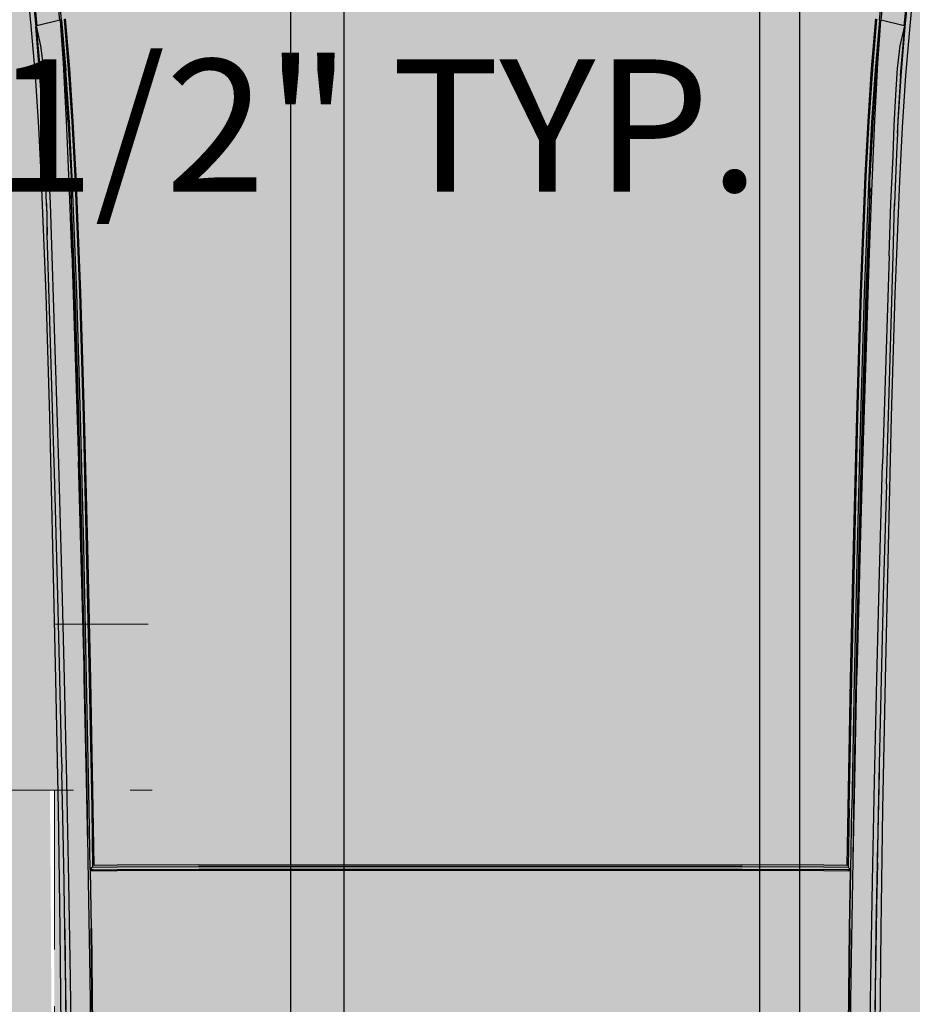
# Model space of a CAD drawing. Units: inches. Extents: x 1884 to 2398, y 474 to 1488.
# Tile 24 of 39: x 2301 to 2348, y 620 to 672. Entities that reach past the tile are written whole.
import ezdxf

# ---------------------------------------------------------------- set-up
doc = ezdxf.new("R2010")
doc.units = ezdxf.units.IN
doc.header["$MEASUREMENT"] = 0
doc.linetypes.add('ACAD_ISO02W100', pattern=[15, 12, -3])
doc.layers.get('0').update_dxf_attribs({"color": 250})
for name, color, linetype, lineweight in [('A-ANNO-DIMS', 2, 'Continuous', 18), ('A-FLOR-OVHD', 8, 'ACAD_ISO02W100', 18), ('C-VEHI', 8, 'Continuous', 18)]:
    doc.layers.add(name, color=color, linetype=linetype, lineweight=lineweight)
doc.layers.add('Edges', color=250, linetype='Continuous')
doc.layers.add('L-PVMT-PATT', color=9, linetype='Continuous', lineweight=13, true_color=0xc7c8ca)
doc.styles.get("Standard").update_dxf_attribs({"font": 'arial.ttf'})
doc.dimstyles.get("Standard").update_dxf_attribs({"dimtxt": 7, "dimasz": 0.18, "dimexe": 0.18, "dimexo": 0.0625, "dimgap": 0.09, "dimtad": 0, "dimtih": 1, "dimtoh": 1, "dimzin": 0, "dimdsep": 46, "dimlunit": 3, "dimtxsty": 'Standard', "dimcen": 0.09, "dimadec": 0, "dimazin": 0, "dimtfac": 1, "dimtofl": 0, "dimtmove": 0, "dimatfit": 3, "dimfxl": 1, "dimtolj": 1, "dimtzin": 0, "dimarcsym": 0})

# ---------------------------------------------------------------- blocks, each defined once
blk = doc.blocks.new('Nissan Qashqai pl')
at = {"layer": 'Edges'}
for p, q in [((9.2783, 12.5191), (9.3422, 12.5126)), ((9.3427, 12.5066), (9.2789, 12.5131)), ((9.3418, 12.5051), (9.2819, 12.5112)), ((9.3418, 12.5051), (9.3346, 12.4741)), ((9.342, 12.5059), (9.3418, 12.5051)), ((9.3687, 12.5), (9.342, 12.5059)), ((9.4087, 12.5003), (9.342, 12.5059)), ((9.3422, 12.5126), (9.4088, 12.507)), ((9.4093, 12.5011), (9.3427, 12.5066)), ((9.4088, 12.507), (9.4782, 12.5024)), ((9.4782, 12.5024), (9.5503, 12.4987)), ((9.3992, 12.496), (9.3687, 12.5)), ((9.4347, 12.494), (9.3992, 12.496)), ((9.4087, 12.5003), (9.4688, 12.4968)), ((9.4785, 12.4965), (9.4093, 12.5011)), ((9.4761, 12.4919), (9.4347, 12.494)), ((9.4688, 12.4968), (9.4789, 12.4964)), ((9.5168, 12.4903), (9.4761, 12.4919)), ((9.4789, 12.4964), (9.4785, 12.4965)), ((9.4862, 12.4961), (9.4785, 12.4965)), ((9.4789, 12.4964), (9.4862, 12.4961)), ((9.4862, 12.4961), (9.514, 12.4949)), ((9.514, 12.4949), (9.5811, 12.492)), ((9.5812, 12.4874), (9.5168, 12.4903)), ((9.5503, 12.4987), (9.7029, 12.4926)), ((9.651, 12.4906), (9.5811, 12.492)), ((9.5811, 12.492), (9.594, 12.4914)), ((9.9583, 12.4812), (9.651, 12.4906)), ((9.7029, 12.4926), (9.8673, 12.4878)), ((9.3346, 12.4718), (9.2704, 12.4783)), ((9.3346, 12.4741), (9.2724, 12.4804)), ((9.6514, 12.4849), (9.5812, 12.4874)), ((9.6514, 12.4849), (9.9312, 12.4761)), ((9.8673, 12.4878), (10.0423, 12.4835)), ((10.0776, 12.4719), (9.9312, 12.4761)), ((9.9583, 12.4812), (10.091, 12.4775)), ((10.0423, 12.4835), (10.2211, 12.4795)), ((10.091, 12.4775), (10.2202, 12.4743)), ((10.2211, 12.4795), (10.3955, 12.4762)), ((10.3955, 12.4762), (10.5572, 12.4737)), ((9.3326, 12.4666), (9.4, 12.4609)), ((9.4004, 12.4629), (9.333, 12.4685)), ((9.3346, 12.4741), (9.3344, 12.4733)), ((9.3344, 12.4733), (9.4017, 12.4677)), ((9.3344, 12.4733), (9.3611, 12.4715)), ((9.3346, 12.4718), (9.4018, 12.4661)), ((9.3611, 12.4715), (9.3918, 12.4695)), ((9.3918, 12.4695), (9.4276, 12.4674)), ((9.4709, 12.4581), (9.4004, 12.4629)), ((9.4017, 12.4677), (9.472, 12.463)), ((9.4018, 12.4661), (9.472, 12.4614)), ((9.4276, 12.4674), (9.4694, 12.4654)), ((9.4694, 12.4654), (9.5105, 12.4637)), ((9.472, 12.463), (9.5454, 12.4591)), ((9.5105, 12.4637), (9.5755, 12.4608)), ((10.2201, 12.4683), (10.0776, 12.4719)), ((10.3586, 12.4651), (10.2201, 12.4683)), ((10.2202, 12.4743), (10.2203, 12.4743)), ((10.2203, 12.4743), (10.3353, 12.4717)), ((10.3353, 12.4717), (10.4477, 12.4694)), ((10.3353, 12.4717), (10.346, 12.4714)), ((10.346, 12.4714), (10.4477, 12.4694)), ((10.4931, 12.4624), (10.3586, 12.4651)), ((10.4477, 12.4694), (10.4538, 12.4693)), ((10.4538, 12.4693), (10.4681, 12.469)), ((10.4676, 12.4691), (10.4538, 12.4693)), ((10.5566, 12.4677), (10.4676, 12.4691)), ((10.4676, 12.4691), (10.546, 12.4677)), ((10.4681, 12.469), (10.5866, 12.467)), ((10.6237, 12.4603), (10.4931, 12.4624)), ((10.546, 12.4677), (10.546, 12.4678)), ((10.546, 12.4677), (10.5576, 12.4675)), ((10.7, 12.4662), (10.5566, 12.4677)), ((10.5572, 12.4737), (10.7004, 12.4722)), ((10.5576, 12.4675), (10.6649, 12.4659)), ((10.5866, 12.467), (10.6649, 12.4659)), ((9.4, 12.4609), (9.4706, 12.4561)), ((9.4706, 12.4561), (9.5443, 12.4522)), ((9.5446, 12.4542), (9.4709, 12.4581)), ((9.472, 12.4614), (9.5454, 12.4576)), ((9.5443, 12.4522), (9.701, 12.4459)), ((9.7011, 12.4478), (9.5446, 12.4542)), ((9.5454, 12.4591), (9.5454, 12.4593)), ((9.5695, 12.4589), (9.5454, 12.4591)), ((9.5454, 12.4576), (9.7014, 12.4513)), ((9.5609, 12.4593), (9.5695, 12.4589)), ((9.5786, 12.4588), (9.5695, 12.4589)), ((9.5695, 12.4589), (9.7014, 12.4536)), ((9.5755, 12.4608), (9.6472, 12.4581)), ((9.6206, 12.4581), (9.5786, 12.4588)), ((9.6714, 12.4567), (9.6206, 12.4581)), ((9.6414, 12.458), (9.6407, 12.458)), ((9.6472, 12.4581), (9.9278, 12.4492)), ((9.6549, 12.4576), (9.6558, 12.4574)), ((9.6825, 12.4564), (9.6714, 12.4567)), ((9.6825, 12.4564), (9.6829, 12.4563)), ((9.6943, 12.456), (9.6825, 12.4564)), ((9.6943, 12.4558), (9.6943, 12.456)), ((9.6951, 12.456), (9.6943, 12.456)), ((9.6951, 12.4558), (9.6951, 12.456)), ((9.8565, 12.451), (9.6951, 12.456)), ((9.7014, 12.4536), (9.8673, 12.4488)), ((9.7014, 12.4513), (9.8673, 12.4464)), ((9.9794, 12.4475), (9.8565, 12.451)), ((9.8673, 12.4488), (10.0429, 12.4444)), ((9.9278, 12.4492), (10.0747, 12.445)), ((10.7502, 12.4586), (10.6237, 12.4603)), ((9.701, 12.4459), (9.8673, 12.441)), ((9.8673, 12.443), (9.7011, 12.4478)), ((9.8673, 12.4464), (10.0429, 12.4421)), ((10.043, 12.4387), (9.8673, 12.443)), ((9.8673, 12.441), (10.0431, 12.4367)), ((10.0998, 12.4443), (9.9794, 12.4475)), ((10.0429, 12.4444), (10.2216, 12.4404)), ((10.0429, 12.4421), (10.2215, 12.4381)), ((10.2218, 12.4347), (10.043, 12.4387)), ((10.0431, 12.4367), (10.2218, 12.4327)), ((10.0747, 12.445), (10.078, 12.4449)), ((10.078, 12.4449), (10.2146, 12.4414)), ((10.2146, 12.4414), (10.0998, 12.4443)), ((10.2146, 12.4414), (10.2175, 12.4413)), ((10.2175, 12.4413), (10.3564, 12.4382)), ((10.2215, 12.4381), (10.3945, 12.4348)), ((10.2216, 12.4404), (10.3947, 12.4371)), ((10.3564, 12.4382), (10.4638, 12.436)), ((10.3947, 12.4371), (10.4638, 12.436)), ((10.4638, 12.436), (10.4914, 12.4355)), ((10.4914, 12.4355), (10.6223, 12.4333)), ((10.3947, 12.4314), (10.2218, 12.4347)), ((10.2218, 12.4327), (10.3947, 12.4294)), ((10.4773, 12.4335), (10.3945, 12.4348)), ((10.3947, 12.4314), (10.4735, 12.4301)), ((10.3947, 12.4294), (10.4715, 12.4282)), ((10.4715, 12.4282), (10.4711, 12.3973)), ((10.4731, 12.3973), (10.4735, 12.4301)), ((10.4735, 12.4301), (10.4773, 12.4335)), ((10.4773, 12.4296), (10.4769, 12.3968)), ((10.4773, 12.4335), (10.4773, 12.4296)), ((10.4785, 12.433), (10.4773, 12.4335)), ((10.5561, 12.4323), (10.4773, 12.4335)), ((10.4781, 12.3972), (10.4785, 12.433)), ((10.5563, 12.4318), (10.4785, 12.433)), ((10.5561, 12.4323), (10.6996, 12.4308)), ((10.6999, 12.4304), (10.5563, 12.4318)), ((10.6223, 12.4333), (10.7493, 12.4316)), ((10.4711, 12.3973), (10.4706, 12.2875)), ((10.4726, 12.2875), (10.4731, 12.3973)), ((10.4764, 12.2872), (10.4769, 12.3968)), ((10.4776, 12.2874), (10.4781, 12.3972)), ((10.4706, 11.5566), (10.4706, 12.2875)), ((10.4726, 11.5567), (10.4726, 12.2875)), ((10.4764, 11.5569), (10.4764, 12.2872)), ((10.4776, 11.5567), (10.4776, 12.2874)), ((10.4706, 11.5566), (10.4711, 11.4469)), ((10.4731, 11.4469), (10.4726, 11.5567)), ((10.4769, 11.4474), (10.4764, 11.5569)), ((10.4781, 11.4469), (10.4776, 11.5567)), ((10.4711, 11.4469), (10.4715, 11.416)), ((10.4735, 11.414), (10.4731, 11.4469)), ((10.4773, 11.4146), (10.4769, 11.4474)), ((10.4785, 11.4111), (10.4781, 11.4469)), ((10.4715, 11.416), (10.3947, 11.4148)), ((9.8673, 11.4031), (9.701, 11.3983)), ((10.0431, 11.4075), (9.8673, 11.4031)), ((9.8673, 11.4012), (10.043, 11.4055)), ((10.2215, 11.406), (10.0429, 11.4021)), ((10.2216, 11.4037), (10.0429, 11.3998)), ((10.043, 11.4055), (10.2218, 11.4094)), ((10.2218, 11.4114), (10.0431, 11.4075)), ((10.2043, 11.4025), (10.0747, 11.3991)), ((10.0998, 11.3999), (10.2043, 11.4025)), ((10.2175, 11.4028), (10.2043, 11.4025)), ((10.3564, 11.406), (10.2175, 11.4028)), ((10.3945, 11.4094), (10.2215, 11.406)), ((10.3947, 11.4071), (10.2216, 11.4037)), ((10.3947, 11.4148), (10.2218, 11.4114)), ((10.2218, 11.4094), (10.3947, 11.4128)), ((10.4416, 11.4077), (10.3564, 11.406)), ((10.4773, 11.4107), (10.3945, 11.4094)), ((10.3947, 11.4128), (10.4735, 11.414)), ((10.4416, 11.4078), (10.3947, 11.4071)), ((10.4519, 11.4079), (10.4416, 11.4077)), ((10.4519, 11.4079), (10.4416, 11.4078)), ((10.4416, 11.4077), (10.4416, 11.4078)), ((10.4524, 11.408), (10.4519, 11.4079)), ((10.4519, 11.4079), (10.4519, 11.4079)), ((10.4524, 11.4079), (10.4519, 11.4079)), ((10.4524, 11.4079), (10.4524, 11.408)), ((10.4533, 11.408), (10.4524, 11.408)), ((10.4533, 11.4079), (10.4524, 11.4079)), ((10.4638, 11.4081), (10.4533, 11.4079)), ((10.4638, 11.4081), (10.4533, 11.408)), ((10.4533, 11.4079), (10.4533, 11.408)), ((10.4914, 11.4087), (10.4638, 11.4081)), ((10.4773, 11.4107), (10.4735, 11.414)), ((10.4773, 11.4146), (10.4773, 11.4107)), ((10.4773, 11.4107), (10.5561, 11.4119)), ((10.4773, 11.4107), (10.4785, 11.4111)), ((10.5563, 11.4123), (10.4785, 11.4111)), ((10.6223, 11.4109), (10.4914, 11.4087)), ((10.6996, 11.4134), (10.5561, 11.4119)), ((10.5563, 11.4123), (10.6999, 11.4138)), ((10.7493, 11.4125), (10.6223, 11.4109)), ((9.5443, 11.3919), (9.4706, 11.388)), ((9.4709, 11.3861), (9.5446, 11.39)), ((9.701, 11.3983), (9.5443, 11.3919)), ((9.5446, 11.39), (9.7011, 11.3963)), ((9.7014, 11.3929), (9.5454, 11.3866)), ((9.7014, 11.3906), (9.5695, 11.3853)), ((9.6472, 11.3861), (9.9278, 11.3949)), ((9.6714, 11.3874), (9.8565, 11.3931)), ((9.7011, 11.3963), (9.8673, 11.4012)), ((9.8673, 11.3977), (9.7014, 11.3929)), ((9.8673, 11.3954), (9.7014, 11.3906)), ((9.8565, 11.3931), (9.9794, 11.3967)), ((10.0429, 11.4021), (9.8673, 11.3977)), ((10.0429, 11.3998), (9.8673, 11.3954)), ((10.0747, 11.3991), (9.9278, 11.3949)), ((9.9794, 11.3967), (10.0965, 11.3998)), ((10.0965, 11.3998), (10.0998, 11.3999)), ((9.4, 11.3832), (9.3326, 11.3776)), ((9.333, 11.3757), (9.4004, 11.3813)), ((9.4017, 11.3765), (9.3344, 11.3708)), ((9.3346, 11.3724), (9.4018, 11.378)), ((9.4276, 11.3767), (9.3918, 11.3747)), ((9.4706, 11.388), (9.4, 11.3832)), ((9.4004, 11.3813), (9.4709, 11.3861)), ((9.472, 11.3812), (9.4017, 11.3765)), ((9.472, 11.3828), (9.4018, 11.378)), ((9.4694, 11.3788), (9.4276, 11.3767)), ((9.5105, 11.3805), (9.4694, 11.3788)), ((9.5454, 11.3866), (9.472, 11.3828)), ((9.472, 11.3812), (9.5454, 11.3851)), ((9.5755, 11.3834), (9.5105, 11.3805)), ((9.5454, 11.3851), (9.5695, 11.3853)), ((9.5454, 11.3848), (9.5454, 11.3851)), ((9.5695, 11.3853), (9.5609, 11.3849)), ((9.5695, 11.3853), (9.5786, 11.3853)), ((9.6472, 11.3861), (9.5755, 11.3834)), ((9.5786, 11.3853), (9.6206, 11.3861)), ((9.6206, 11.3861), (9.6714, 11.3874)), ((10.0776, 11.3722), (10.2201, 11.3759)), ((10.2201, 11.3759), (10.3586, 11.3791)), ((10.3586, 11.3791), (10.4931, 11.3817)), ((10.5576, 11.3766), (10.4676, 11.3751)), ((10.5566, 11.3765), (10.4676, 11.3751)), ((10.5866, 11.3772), (10.4681, 11.3752)), ((10.4931, 11.3817), (10.6237, 11.3839)), ((10.5566, 11.3765), (10.7, 11.378)), ((10.6649, 11.3783), (10.5576, 11.3766)), ((10.6649, 11.3783), (10.5866, 11.3772)), ((10.6237, 11.3839), (10.7502, 11.3855)), ((9.3346, 11.3724), (9.2704, 11.3659)), ((9.3346, 11.37), (9.2724, 11.3637)), ((9.3611, 11.3727), (9.3344, 11.3708)), ((9.3344, 11.3708), (9.3346, 11.37)), ((9.3346, 11.37), (9.3418, 11.3391)), ((9.3918, 11.3747), (9.3611, 11.3727)), ((9.9583, 11.363), (9.651, 11.3536)), ((9.6514, 11.3592), (9.9312, 11.3681)), ((9.9312, 11.3681), (10.0776, 11.3722)), ((10.091, 11.3666), (9.9583, 11.363)), ((10.2211, 11.3646), (10.0423, 11.3607)), ((10.2191, 11.3699), (10.091, 11.3666)), ((10.2202, 11.3699), (10.2191, 11.3699)), ((10.2202, 11.3699), (10.2203, 11.3699)), ((10.3353, 11.3725), (10.2203, 11.3699)), ((10.3955, 11.368), (10.2211, 11.3646)), ((10.3353, 11.3725), (10.346, 11.3727)), ((10.4477, 11.3747), (10.346, 11.3727)), ((10.5572, 11.3704), (10.3955, 11.368)), ((10.4537, 11.3749), (10.4477, 11.3747)), ((10.4537, 11.3749), (10.4538, 11.3749)), ((10.4681, 11.3752), (10.4538, 11.3749)), ((10.4676, 11.3751), (10.4538, 11.3749)), ((10.4676, 11.3751), (10.4676, 11.3751)), ((10.7004, 11.372), (10.5572, 11.3704)), ((9.3992, 11.3482), (9.4347, 11.3502)), ((9.4347, 11.3502), (9.4761, 11.3522)), ((9.4761, 11.3522), (9.5168, 11.3539)), ((9.5811, 11.3522), (9.514, 11.3492)), ((9.5168, 11.3539), (9.5812, 11.3568)), ((9.7029, 11.3516), (9.5503, 11.3455)), ((9.5811, 11.3522), (9.6231, 11.3531)), ((9.594, 11.3527), (9.5811, 11.3522)), ((9.5812, 11.3568), (9.6514, 11.3592)), ((9.6231, 11.3531), (9.594, 11.3527)), ((9.651, 11.3536), (9.6231, 11.3531)), ((9.8673, 11.3563), (9.7029, 11.3516)), ((10.0423, 11.3607), (9.8673, 11.3563)), ((9.2789, 11.331), (9.3427, 11.3375)), ((9.2819, 11.333), (9.3418, 11.3391)), ((9.3418, 11.3391), (9.342, 11.3383)), ((9.342, 11.3383), (9.3687, 11.3441)), ((9.342, 11.3383), (9.4087, 11.3438)), ((9.4088, 11.3371), (9.3422, 11.3316)), ((9.4093, 11.3431), (9.3427, 11.3375)), ((9.3687, 11.3441), (9.3992, 11.3482)), ((9.4605, 11.3465), (9.4087, 11.3438)), ((9.4782, 11.3418), (9.4088, 11.3371)), ((9.4605, 11.3465), (9.4093, 11.3431)), ((9.514, 11.3492), (9.4605, 11.3465)), ((9.5503, 11.3455), (9.4782, 11.3418)), ((9.3422, 11.3316), (9.2783, 11.3251))]:
    blk.add_line(p, q, dxfattribs=at)
blk = doc.blocks.new('car')
blk.add_blockref('Nissan Qashqai pl', (-9.7433, -11.9151))
blk = doc.blocks.new('carr')
blk.add_blockref('car', (0.5124, -0.007))
blk = doc.blocks.new('*D23')
at = {"layer": 'A-ANNO-DIMS', "color": 0, "lineweight": -2, "transparency": 16777216}
for p, q in [((2272.304, 752.812), (2298.291, 752.812)), ((2298.111, 752.632), (2298.111, 670.29)), ((2298.111, 580.529), (2298.111, 662.871)), ((2272.304, 580.349), (2298.291, 580.349))]:
    blk.add_line(p, q, dxfattribs=at)
at = {"layer": 'A-ANNO-DIMS', "color": 0, "lineweight": 100, "transparency": 16777216}
for points in [[(2298.081, 752.632), (2298.141, 752.632), (2298.111, 752.812)], [(2298.081, 580.529), (2298.141, 580.529), (2298.111, 580.349)]]:
    blk.add_solid(points, dxfattribs=at)
at = {"layer": 'Defpoints', "color": 0, "lineweight": 100, "transparency": 16777216}
for p in [(2272.242, 752.812), (2272.242, 580.349), (2298.111, 580.349)]:
    blk.add_point(p, dxfattribs=at)
at = {"layer": 'A-ANNO-DIMS', "color": 0, "transparency": 16777216, "insert": (2298.111, 666.58), "char_height": 7, "attachment_point": 5}
blk.add_mtext('\\A1;CAR 14\'-4 1/2" TYP.', dxfattribs=at)
blk = doc.blocks.new('*D47')
at = {"layer": 'A-ANNO-DIMS', "color": 0, "lineweight": -2, "transparency": 16777216}
for p, q in [((2315.591, 959.704), (2315.591, 484.005)), ((2342.529, 959.704), (2342.529, 484.005)), ((2315.771, 484.185), (2319.606, 484.185)), ((2342.349, 484.185), (2338.513, 484.185))]:
    blk.add_line(p, q, dxfattribs=at)
at = {"layer": 'A-ANNO-DIMS', "color": 0, "lineweight": 100, "transparency": 16777216}
for points in [[(2315.771, 484.215), (2315.771, 484.155), (2315.591, 484.185)], [(2342.349, 484.215), (2342.349, 484.155), (2342.529, 484.185)]]:
    blk.add_solid(points, dxfattribs=at)
at = {"layer": 'Defpoints', "color": 0, "lineweight": 100, "transparency": 16777216}
for p in [(2315.591, 959.766), (2342.529, 959.766), (2342.529, 484.185)]:
    blk.add_point(p, dxfattribs=at)
at = {"layer": 'A-ANNO-DIMS', "color": 0, "transparency": 16777216, "insert": (2329.06, 484.185), "char_height": 7, "attachment_point": 5}
blk.add_mtext('\\A1;2\'-3"', dxfattribs=at)
blk = doc.blocks.new('*D49')
at = {"layer": 'A-ANNO-DIMS', "color": 0, "lineweight": -2, "transparency": 16777216}
for p, q in [((2318.409, 987.716), (2318.409, 484.005)), ((2340.409, 987.716), (2340.409, 484.005)), ((2318.589, 484.185), (2340.229, 484.185)), ((2340.409, 484.185), (2340.589, 484.185))]:
    blk.add_line(p, q, dxfattribs=at)
at = {"layer": 'A-ANNO-DIMS', "color": 0, "lineweight": 100, "transparency": 16777216}
for points in [[(2318.589, 484.215), (2318.589, 484.155), (2318.409, 484.185)], [(2340.229, 484.215), (2340.229, 484.155), (2340.409, 484.185)]]:
    blk.add_solid(points, dxfattribs=at)
at = {"layer": 'Defpoints', "color": 0, "lineweight": 100, "transparency": 16777216}
for p in [(2318.409, 987.778), (2340.409, 987.778), (2340.409, 484.185)]:
    blk.add_point(p, dxfattribs=at)
at = {"layer": 'A-ANNO-DIMS', "color": 0, "transparency": 16777216, "insert": (2352.373, 484.185), "char_height": 7, "attachment_point": 5}
blk.add_mtext('\\A1;1\'-10"', dxfattribs=at)

msp = doc.modelspace()

# ---------------------------------------------------------------- hatches: boundary and pattern name
at = {"layer": 'L-PVMT-PATT'}
h = msp.add_hatch(color=256, dxfattribs=at)
h.dxf.hatch_style = 1
h.paths.add_polyline_path([(2387.529, 769.966), (2351.529, 769.966), (2238.447, 769.966), (2238.447, 762.15), (2238.447, 754.445), (2126.529, 754.445), (2126.529, 676.183), (2134.868, 676.183), (2142.673, 676.183), (2142.673, 646.578), (2134.868, 646.578), (2126.529, 646.578), (2126.529, 640.17), (2387.529, 640.17)])
h.paths.add_polyline_path([(2387.529, 631.385), (2303.086, 631.385), (2303.086, 615.671), (2387.529, 615.671)])
h.paths.add_polyline_path([(2387.529, 640.17), (2126.529, 640.17), (2126.529, 631.385), (2387.529, 631.385)])
h.paths.add_polyline_path([(2393.529, 604.13), (2387.529, 604.13), (2387.529, 615.671), (2303.086, 615.671), (2303.086, 607.943), (2249.649, 607.943), (2126.529, 607.943), (2126.529, 533.885), (2393.529, 533.885)])
h.paths.add_polyline_path([(2257.825, 611.008), (2257.83, 611.337), (2257.915, 616.493), (2258.021, 621.805), (2258.146, 627.274), (2258.252, 631.385), (2126.529, 631.385), (2126.529, 611.008)])
h.paths.add_polyline_path([(2258.892, 611.285), (2258.888, 611.008), (2300.247, 611.008), (2300.247, 631.385), (2259.314, 631.385), (2259.206, 627.173), (2259.081, 621.72), (2258.976, 616.424)])
h = msp.add_hatch(color=256, dxfattribs=at)
h.dxf.hatch_style = 1
h.paths.add_polyline_path([(2216.015, 611.008), (2212.351, 611.008), (2212.342, 608.327), (2212.34, 607.943), (2216.046, 607.943), (2216.044, 608.264)])
h.paths.add_polyline_path([(2212.351, 611.008), (2211.081, 611.008), (2210.074, 609.575), (2209.435, 608.376), (2209.305, 607.943), (2212.34, 607.943), (2212.342, 608.327)])
h.paths.add_polyline_path([(2257.742, 611.008), (2249.649, 611.008), (2217.664, 611.008), (2217.692, 608.284), (2217.694, 607.943), (2249.649, 607.943), (2257.712, 607.943), (2257.713, 608.284)])
h.paths.add_polyline_path([(2266.79, 611.008), (2264.592, 611.008), (2265.355, 609.923), (2266.022, 608.672), (2266.241, 607.943), (2266.364, 607.943), (2266.622, 609.602)])
h.paths.add_polyline_path([(2263.055, 611.008), (2259.39, 611.008), (2259.361, 608.264), (2259.359, 607.943), (2263.065, 607.943), (2263.063, 608.327)])
h.paths.add_polyline_path([(2265.331, 609.575), (2264.325, 611.008), (2263.055, 611.008), (2263.063, 608.327), (2263.065, 607.943), (2266.1, 607.943), (2265.97, 608.376)])
h.paths.add_polyline_path([(2272.885, 609.347), (2272.901, 609.457), (2272.902, 609.679), (2272.895, 611.008), (2271.456, 611.008), (2271.351, 610.147), (2271.277, 610.077), (2270.912, 610.081), (2270.481, 610.11), (2270.455, 610.183), (2270.448, 611.008), (2269.23, 611.008), (2269.228, 610.963), (2269.055, 608.458), (2269.014, 607.943), (2272.869, 607.943), (2272.882, 607.958)])
h.paths.add_polyline_path([(2269.228, 610.963), (2269.23, 611.008), (2267.227, 611.008), (2267.038, 609.547), (2266.77, 607.943), (2269.014, 607.943), (2269.055, 608.458)])
h.paths.add_polyline_path([(2293.178, 611.008), (2272.917, 611.008), (2272.925, 609.643), (2272.924, 609.184), (2272.925, 609.03), (2272.921, 607.943), (2293.123, 607.943), (2293.127, 608.565), (2293.159, 610.362)])
h.paths.add_polyline_path([(2302.932, 613.651), (2302.931, 615.98), (2302.91, 623.22), (2302.851, 630.905), (2302.844, 631.385), (2300.247, 631.385), (2300.247, 612.163), (2300.885, 611.925), (2301.121, 611.86), (2301.743, 612.576)])
h.paths.add_polyline_path([(2302.992, 610.861), (2302.993, 612.796), (2302.965, 612.8), (2301.576, 611.546), (2300.954, 610.83), (2300.899, 610.766), (2300.444, 610.894), (2300.139, 611.008), (2299.369, 611.008), (2299.448, 609.776), (2299.311, 611.008), (2299.207, 611.008), (2299.34, 609.722), (2299.553, 607.943), (2300.825, 607.943), (2300.851, 607.993), (2301.87, 609.442)])
h.paths.add_polyline_path([(2298.512, 611.008), (2296.882, 611.008), (2296.979, 609.034), (2297.054, 607.943), (2298.828, 607.943), (2298.736, 608.659)])
h.paths.add_polyline_path([(2294.51, 608.662), (2294.51, 608.662), (2294.362, 610.672), (2294.359, 611.008), (2293.338, 611.008), (2293.331, 610.606), (2293.329, 610.538), (2293.315, 609.691), (2293.305, 607.943), (2294.597, 607.943)])
h.paths.add_polyline_path([(2302.991, 609.68), (2301.718, 608.051), (2301.642, 607.943), (2302.986, 607.943)], flags=17)

# ---------------------------------------------------------------- linework, layer by layer
at = {"layer": 'A-FLOR-OVHD'}
for p, q in [((2258.112, 640.17), (2308.043, 640.17)), ((2262.087, 631.385), (2308.262, 631.385)), ((2303.086, 607.943), (2303.086, 631.385))]:
    msp.add_line(p, q, dxfattribs=at)

# ---------------------------------------------------------------- block references
at = {"layer": 'C-VEHI', "xscale": 39.37007874015748, "yscale": 39.37007874015748, "zscale": 39.37007874015748, "rotation": 270}
msp.add_blockref('carr', (2325.111, 676.232), dxfattribs=at)

# ---------------------------------------------------------------- dimensions: what is measured, and where the dimension line sits
at = {"layer": 'A-ANNO-DIMS'}
for base, p1, p2, picture, middle in [((2340.409, 484.185), (2318.409, 987.778), (2340.409, 987.778), '*D49', (2352.373, 484.185)), ((2342.529, 484.185), (2315.591, 959.766), (2342.529, 959.766), '*D47', (2329.06, 484.185))]:
    dim = msp.add_linear_dim(base=base, p1=p1, p2=p2, dimstyle='Standard', override={"dimdec": 1, "dimlfac": 1, "dimrnd": 0, "dimzin": 1, "dimdsep": 46, "dimlunit": 4, "dimfrac": 2}, dxfattribs=at)
    dim.commit()
    dim.dimension.update_dxf_attribs({"geometry": picture, "text_midpoint": middle})
dim = msp.add_linear_dim(base=(2298.111, 580.349), p1=(2272.242, 752.812), p2=(2272.242, 580.349), angle=270, text='CAR <> TYP.', dimstyle='Standard', override={"dimdec": 1, "dimlfac": 1, "dimrnd": 0, "dimzin": 1, "dimdsep": 46, "dimlunit": 4, "dimfrac": 2}, dxfattribs=at)
dim.commit()
dim.dimension.update_dxf_attribs({"geometry": '*D23', "text_midpoint": (2298.111, 666.58)})

doc.saveas('drawing.dxf')
